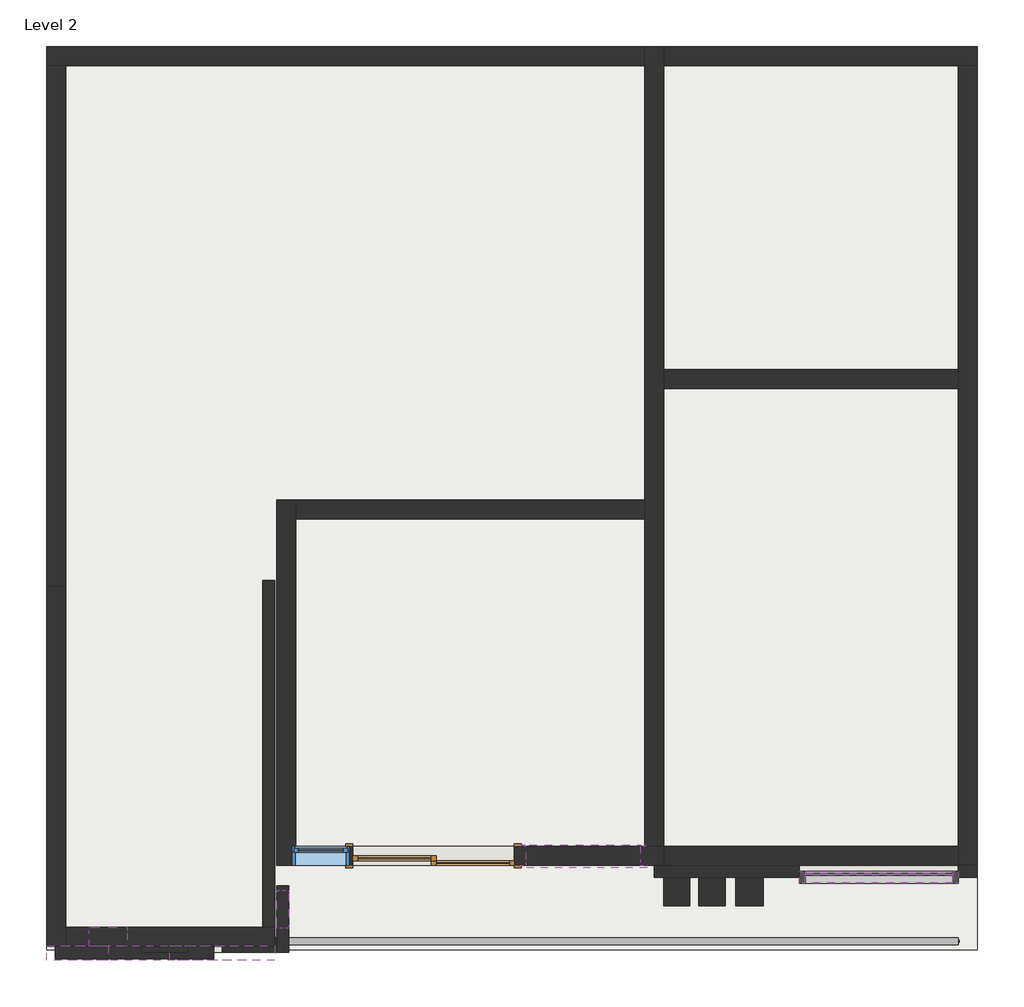
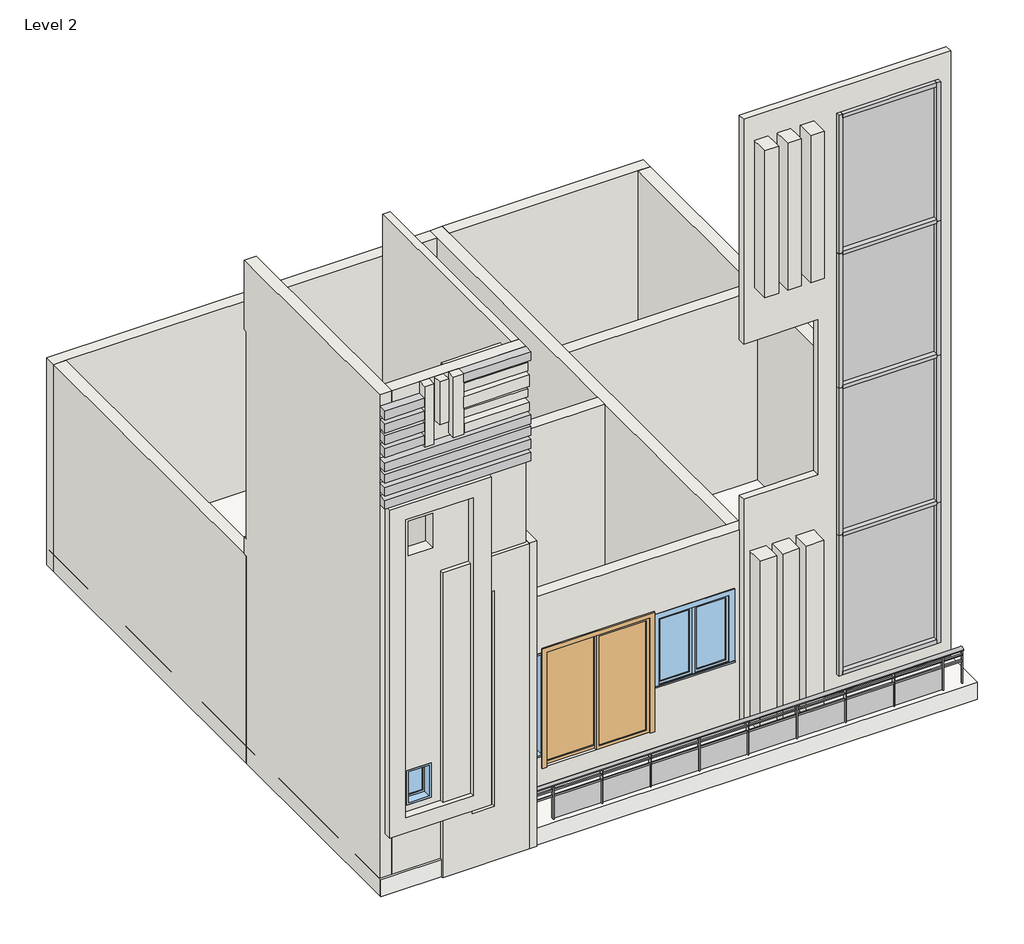
# One storey: 18 walls, 13 members, 9 proxies, 4 plates, 4 windows, 1 door, 1 railing, 1 roof.
"""IFC4 building model written with IfcOpenShell, lengths in millimetres."""

from ifc_helpers import new_model, si_unit, point, frame, origin, place, context, project, spatial, polyline, ellipse_curve, trimmed, outline, extrude, faceted_brep, transform, mapped, element, save
from ifc_brep_helpers import plane_surface, extruded_surface, advanced_brep
from components import door_076b30e0, member_15dc5290, member_cf032248, member_591cd9a7, member_6ce1ec76, member_029677a6, member_d6a8c742, system_panel_glazed_8270a400, system_panel_glazed_e50b416a, system_panel_glazed_3bb4e025, system_panel_glazed_87f78641, walls_3_walls_3_caf9bd33, walls_4_walls_4_15621a10, window_0862ab64, window_085f26e1, window_f83fec05, window_50feeedf

model = new_model("IFC4")

# Units and contexts
model_context = context("Model", 3, world=origin())
ifc_project = project(units=[si_unit("LENGTHUNIT", "METRE", prefix="MILLI")], contexts=[model_context])

# Site, building, storey
site = spatial("IfcSite", under=ifc_project)
building = spatial("IfcBuilding", under=site)
storey = spatial("IfcBuildingStorey", under=building, Name="Level 2", Elevation=3657.6)

# Proxies
placement = place(None, origin())
element("IfcBuildingElementProxy", 1, Name="Cornice", ObjectType="Cornice", at=placement, inside=storey, context=model_context, shape_type="SweptSolid", body=[
    extrude(outline(polyline([(-10979.7013569, 231.2548743), (-10979.7013569, 383.6548743), (-9861.3432037, 383.6548743), (-9861.3432037, 231.2548743), (-10979.7013569, 231.2548743)])), frame((0.0, 0.0, 12344.4), z_axis=(0.0, 0.0, 1.0), x_axis=(1.0, 0.0, 0.0)), (0.0, 0.0, 1.0), 152.4),
])
element("IfcBuildingElementProxy", 2, Name="Cornice", ObjectType="Cornice", at=placement, inside=storey, context=model_context, shape_type="SweptSolid", body=[
    extrude(outline(polyline([(-12299.7432037, 231.2548743), (-12299.7432037, 383.6548743), (-9861.3432037, 383.6548743), (-9861.3432037, 231.2548743), (-12299.7432037, 231.2548743)])), frame((0.0, 0.0, 11226.8), z_axis=(0.0, 0.0, 1.0), x_axis=(1.0, 0.0, 0.0)), (0.0, 0.0, 1.0), 152.4),
])
element("IfcBuildingElementProxy", 3, Name="Cornice", ObjectType="Cornice", at=placement, inside=storey, context=model_context, shape_type="SweptSolid", body=[
    extrude(outline(polyline([(-12299.7432037, 231.2548743), (-12299.7432037, 383.6548743), (-9861.3432037, 383.6548743), (-9861.3432037, 231.2548743), (-12299.7432037, 231.2548743)])), frame((0.0, 0.0, 11023.6), z_axis=(0.0, 0.0, 1.0), x_axis=(1.0, 0.0, 0.0)), (0.0, 0.0, 1.0), 152.4),
])
element("IfcBuildingElementProxy", 4, Name="Cornice", ObjectType="Cornice", at=placement, inside=storey, context=model_context, shape_type="SweptSolid", body=[
    extrude(outline(polyline([(-12299.7432037, 231.2548743), (-12299.7432037, 383.6548743), (-9861.3432037, 383.6548743), (-9861.3432037, 231.2548743), (-12299.7432037, 231.2548743)])), frame((0.0, 0.0, 10795.0), z_axis=(0.0, 0.0, 1.0), x_axis=(1.0, 0.0, 0.0)), (0.0, 0.0, 1.0), 152.4),
])
element("IfcBuildingElementProxy", 5, Name="Cornice", ObjectType="Cornice", at=placement, inside=storey, context=model_context, shape_type="SweptSolid", body=[
    extrude(outline(polyline([(-12299.7432037, 231.2548743), (-12299.7432037, 383.6548743), (-9861.3432037, 383.6548743), (-9861.3432037, 231.2548743), (-12299.7432037, 231.2548743)])), frame((0.0, 0.0, 10566.4), z_axis=(0.0, 0.0, 1.0), x_axis=(1.0, 0.0, 0.0)), (0.0, 0.0, 1.0), 152.4),
])
element("IfcBuildingElementProxy", 6, Name="Cornice", ObjectType="Cornice", at=placement, inside=storey, context=model_context, shape_type="SweptSolid", body=[
    extrude(outline(polyline([(-12299.7432037, 231.2548743), (-12299.7432037, 383.6548743), (-11639.3432037, 383.6548743), (-11639.3432037, 231.2548743), (-12299.7432037, 231.2548743)])), frame((0.0, 0.0, 11480.8), z_axis=(0.0, 0.0, 1.0), x_axis=(1.0, 0.0, 0.0)), (0.0, 0.0, 1.0), 152.4),
])
element("IfcBuildingElementProxy", 7, Name="Cornice", ObjectType="Cornice", at=placement, inside=storey, context=model_context, shape_type="SweptSolid", body=[
    extrude(outline(polyline([(-12299.7432037, 231.2548743), (-12299.7432037, 383.6548743), (-11639.3432037, 383.6548743), (-11639.3432037, 231.2548743), (-12299.7432037, 231.2548743)])), frame((0.0, 0.0, 11709.4), z_axis=(0.0, 0.0, 1.0), x_axis=(1.0, 0.0, 0.0)), (0.0, 0.0, 1.0), 152.4),
])
element("IfcBuildingElementProxy", 8, Name="Cornice", ObjectType="Cornice", at=placement, inside=storey, context=model_context, shape_type="SweptSolid", body=[
    extrude(outline(polyline([(-12299.7432037, 231.2548743), (-12299.7432037, 383.6548743), (-11639.3432037, 383.6548743), (-11639.3432037, 231.2548743), (-12299.7432037, 231.2548743)])), frame((0.0, 0.0, 11912.6), z_axis=(0.0, 0.0, 1.0), x_axis=(1.0, 0.0, 0.0)), (0.0, 0.0, 1.0), 152.4),
])
element("IfcBuildingElementProxy", 9, Name="Cornice", ObjectType="Cornice", at=placement, inside=storey, context=model_context, shape_type="SweptSolid", body=[
    extrude(outline(polyline([(-12299.7432037, 231.2548743), (-12299.7432037, 383.6548743), (-11639.3432037, 383.6548743), (-11639.3432037, 231.2548743), (-12299.7432037, 231.2548743)])), frame((0.0, 0.0, 12141.2), z_axis=(0.0, 0.0, 1.0), x_axis=(1.0, 0.0, 0.0)), (0.0, 0.0, 1.0), 152.4),
])

# Door
door_shape = door_076b30e0(model_context)
element("IfcDoor", 10, ObjectType="Door-Double-Sliding : 68\" x 80\"", at=placement, inside=storey, context=model_context, shape_type="MappedRepresentation", body=[
    mapped(door_shape, transform((-8159.5432037, 1475.8548743, 4267.2), x_axis=(-1.0, 0.0, 0.0), y_axis=(0.0, -1.0, 0.0), z_axis=(0.0, 0.0, 1.0))),
])

# Members
member_shape = member_15dc5290(model_context)
element("IfcMember", 11, ObjectType="Rectangular Mullion : 2.5\" x 5\" rectangular", at=placement, inside=storey, context=model_context, shape_type="MappedRepresentation", body=[
    mapped(member_shape, transform((-4247.9432037, 1120.2548743, 11750.8760868), x_axis=(-1.0, 0.0, 0.0), y_axis=(0.0, -1.0, 0.0), z_axis=(0.0, 0.0, 1.0))),
])
member_2_shape = member_cf032248(model_context)
element("IfcMember", 12, ObjectType="Rectangular Mullion : 2.5\" x 5\" rectangular", at=placement, inside=storey, context=model_context, shape_type="MappedRepresentation", body=[
    mapped(member_2_shape, transform((-4247.9432037, 1120.2548743, 9380.6380434), x_axis=(-1.0, 0.0, 0.0), y_axis=(0.0, -1.0, 0.0), z_axis=(0.0, 0.0, 1.0))),
])
member_3_shape = member_591cd9a7(model_context)
element("IfcMember", 13, ObjectType="Rectangular Mullion : 2.5\" x 5\" rectangular", at=placement, inside=storey, context=model_context, shape_type="MappedRepresentation", body=[
    mapped(member_3_shape, transform((-2609.6432037, 1120.2548743, 11750.8760868), x_axis=(0.0, 0.0, 1.0), y_axis=(0.0, -1.0, 0.0), z_axis=(1.0, 0.0, 0.0))),
])
element("IfcMember", 14, ObjectType="Rectangular Mullion : 2.5\" x 5\" rectangular", at=placement, inside=storey, context=model_context, shape_type="MappedRepresentation", body=[
    mapped(member_3_shape, transform((-2609.6432037, 1120.2548743, 9380.6380434), x_axis=(0.0, 0.0, 1.0), y_axis=(0.0, -1.0, 0.0), z_axis=(1.0, 0.0, 0.0))),
])
element("IfcMember", 15, ObjectType="Rectangular Mullion : 2.5\" x 5\" rectangular", at=placement, inside=storey, context=model_context, shape_type="MappedRepresentation", body=[
    mapped(member_3_shape, transform((-2609.6432037, 1120.2548743, 6781.8), x_axis=(0.0, 0.0, 1.0), y_axis=(0.0, -1.0, 0.0), z_axis=(1.0, 0.0, 0.0))),
])
element("IfcMember", 16, ObjectType="Rectangular Mullion : 2.5\" x 5\" rectangular", at=placement, inside=storey, context=model_context, shape_type="MappedRepresentation", body=[
    mapped(member_shape, transform((-2546.1432037, 1120.2548743, 9380.6380434), x_axis=(1.0, 0.0, 0.0), y_axis=(0.0, -1.0, 0.0), z_axis=(0.0, 0.0, -1.0))),
])
element("IfcMember", 17, ObjectType="Rectangular Mullion : 2.5\" x 5\" rectangular", at=placement, inside=storey, context=model_context, shape_type="MappedRepresentation", body=[
    mapped(member_2_shape, transform((-2546.1432037, 1120.2548743, 6781.8), x_axis=(1.0, 0.0, 0.0), y_axis=(0.0, -1.0, 0.0), z_axis=(0.0, 0.0, -1.0))),
])
member_4_shape = member_6ce1ec76(model_context)
element("IfcMember", 18, ObjectType="Rectangular Mullion : 2.5\" x 5\" rectangular", at=placement, inside=storey, context=model_context, shape_type="MappedRepresentation", body=[
    mapped(member_4_shape, transform((-4184.4432037, 1120.2548743, 4304.5775678), x_axis=(0.0, 0.0, -1.0), y_axis=(0.0, -1.0, 0.0), z_axis=(-1.0, 0.0, 0.0))),
])
member_5_shape = member_029677a6(model_context)
element("IfcMember", 19, ObjectType="Rectangular Mullion : 2.5\" x 5\" rectangular", at=placement, inside=storey, context=model_context, shape_type="MappedRepresentation", body=[
    mapped(member_5_shape, transform((-4247.9432037, 1120.2548743, 6781.8), x_axis=(-1.0, 0.0, 0.0), y_axis=(0.0, -1.0, 0.0), z_axis=(0.0, 0.0, 1.0))),
])
element("IfcMember", 20, ObjectType="Rectangular Mullion : 2.5\" x 5\" rectangular", at=placement, inside=storey, context=model_context, shape_type="MappedRepresentation", body=[
    mapped(member_5_shape, transform((-2546.1432037, 1120.2548743, 4304.5775678), x_axis=(1.0, 0.0, 0.0), y_axis=(0.0, -1.0, 0.0), z_axis=(0.0, 0.0, -1.0))),
])
element("IfcMember", 21, ObjectType="Rectangular Mullion : 2.5\" x 5\" rectangular", at=placement, inside=storey, context=model_context, shape_type="MappedRepresentation", body=[
    mapped(member_4_shape, transform((-2609.6432037, 1120.2548743, 14197.3141302), x_axis=(0.0, 0.0, 1.0), y_axis=(0.0, -1.0, 0.0), z_axis=(1.0, 0.0, 0.0))),
])
member_6_shape = member_d6a8c742(model_context)
element("IfcMember", 22, ObjectType="Rectangular Mullion : 2.5\" x 5\" rectangular", at=placement, inside=storey, context=model_context, shape_type="MappedRepresentation", body=[
    mapped(member_6_shape, transform((-4247.9432037, 1120.2548743, 14197.3141302), x_axis=(-1.0, 0.0, 0.0), y_axis=(0.0, -1.0, 0.0), z_axis=(0.0, 0.0, 1.0))),
])
element("IfcMember", 23, ObjectType="Rectangular Mullion : 2.5\" x 5\" rectangular", at=placement, inside=storey, context=model_context, shape_type="MappedRepresentation", body=[
    mapped(member_6_shape, transform((-2546.1432037, 1120.2548743, 11750.8760868), x_axis=(1.0, 0.0, 0.0), y_axis=(0.0, -1.0, 0.0), z_axis=(0.0, 0.0, -1.0))),
])

# Plates
system_panel_glazed_shape = system_panel_glazed_8270a400(model_context)
element("IfcPlate", 24, ObjectType="System Panel : Glazed", at=placement, inside=storey, context=model_context, shape_type="MappedRepresentation", body=[
    mapped(system_panel_glazed_shape, transform((-3397.0432037, 1120.2548743, 6813.55), x_axis=(1.0, 0.0, 0.0), y_axis=(0.0, 1.0, 0.0), z_axis=(0.0, 0.0, 1.0))),
])
system_panel_glazed_2_shape = system_panel_glazed_e50b416a(model_context)
element("IfcPlate", 25, ObjectType="System Panel : Glazed", at=placement, inside=storey, context=model_context, shape_type="MappedRepresentation", body=[
    mapped(system_panel_glazed_2_shape, transform((-3397.0432037, 1120.2548743, 9412.3880434), x_axis=(1.0, 0.0, 0.0), y_axis=(0.0, 1.0, 0.0), z_axis=(0.0, 0.0, 1.0))),
])
system_panel_glazed_3_shape = system_panel_glazed_3bb4e025(model_context)
element("IfcPlate", 26, ObjectType="System Panel : Glazed", at=placement, inside=storey, context=model_context, shape_type="MappedRepresentation", body=[
    mapped(system_panel_glazed_3_shape, transform((-3397.0432037, 1120.2548743, 4368.0775678), x_axis=(1.0, 0.0, 0.0), y_axis=(0.0, 1.0, 0.0), z_axis=(0.0, 0.0, 1.0))),
])
system_panel_glazed_4_shape = system_panel_glazed_87f78641(model_context)
element("IfcPlate", 27, ObjectType="System Panel : Glazed", at=placement, inside=storey, context=model_context, shape_type="MappedRepresentation", body=[
    mapped(system_panel_glazed_4_shape, transform((-3397.0432037, 1120.2548743, 11782.6260868), x_axis=(1.0, 0.0, 0.0), y_axis=(0.0, 1.0, 0.0), z_axis=(0.0, 0.0, 1.0))),
])

# Railing
element("IfcRailing", 28, ObjectType="Glass Panel - Bottom Fill", at=placement, inside=storey, context=model_context, shape_type="SolidModel", body=[
    advanced_brep(
    [(-9708.9432037, 472.5548476, 4572.0), (-9708.9432037, 396.3548476, 4572.0), (-2546.1432037, 472.5548476, 4572.0), (-2546.1432037, 396.3548476, 4572.0)],
    [
        (0, 1, ellipse_curve(frame((-9708.9432037, 434.4548476, 4572.0), z_axis=(-1.0, 0.0, 0.0), x_axis=(0.0, -1.0, 0.0)), 38.1, 28.575)),
        (1, 0, ellipse_curve(frame((-9708.9432037, 434.4548476, 4572.0), z_axis=(-1.0, 0.0, 0.0), x_axis=(0.0, -1.0, 0.0)), 38.1, 28.575)),
        (2, 3, ellipse_curve(frame((-2546.1432037, 434.4548476, 4572.0), z_axis=(1.0, 0.0, 0.0), x_axis=(0.0, -1.0, 0.0)), 38.1, 28.575)),
        (3, 2, ellipse_curve(frame((-2546.1432037, 434.4548476, 4572.0), z_axis=(1.0, 0.0, 0.0), x_axis=(0.0, -1.0, 0.0)), 38.1, 28.575)),
        (0, 2),
        (3, 1),
    ],
    [
        plane_surface(frame((-9708.9432037, 434.4548476, 4572.0), z_axis=(-1.0, 0.0, 0.0), x_axis=(0.0, 1.0, 0.0))),
        plane_surface(frame((-2546.1432037, 434.4548476, 4572.0), z_axis=(1.0, 0.0, 0.0), x_axis=(0.0, 1.0, 0.0))),
        extruded_surface(trimmed(ellipse_curve(frame((-2546.1432037, 434.4548476, 4572.0), z_axis=(-1.0, 0.0, 0.0), x_axis=(0.0, -1.0, 0.0)), 38.1, 28.575), [point((-2546.1432037, 472.5548476, 4572.0))], [point((-2546.1432037, 396.3548476, 4572.0))], True, "CARTESIAN"), (-7162.800000000001, 0.0, 0.0), 7162.800000000001),
        extruded_surface(trimmed(ellipse_curve(frame((-2546.1432037, 434.4548476, 4572.0), z_axis=(-1.0, 0.0, 0.0), x_axis=(0.0, -1.0, 0.0)), 38.1, 28.575), [point((-2546.1432037, 396.3548476, 4572.0))], [point((-2546.1432037, 472.5548476, 4572.0))], True, "CARTESIAN"), (-7162.800000000001, 0.0, 0.0), 7162.800000000001),
    ],
    [
        (0, [[1, 2]]),
        (1, [[3, 4]]),
        (2, [[-1, 5, -4, 6]]),
        (3, [[-2, -6, -3, -5]]),
    ],
),
    extrude(outline(polyline([(-9708.9432037, 421.7548476), (-9708.9432037, 447.1548476), (-2546.1432037, 447.1548476), (-2546.1432037, 421.7548476), (-9708.9432037, 421.7548476)])), frame((0.0, 0.0, 4457.7), z_axis=(0.0, 0.0, 1.0), x_axis=(1.0, 0.0, 0.0)), (0.0, 0.0, 1.0), 25.4),
    extrude(outline(polyline([(-9708.9432037, 421.7548476), (-9708.9432037, 447.1548476), (-2546.1432037, 447.1548476), (-2546.1432037, 421.7548476), (-9708.9432037, 421.7548476)])), frame((0.0, 0.0, 4356.1), z_axis=(0.0, 0.0, 1.0), x_axis=(1.0, 0.0, 0.0)), (0.0, 0.0, 1.0), 25.4),
    extrude(outline(polyline([(-2882.6932037, 409.0548476), (-2882.6932037, 459.8548476), (-2869.9932037, 459.8548476), (-2869.9932037, 409.0548476), (-2882.6932037, 409.0548476)])), frame((0.0, 0.0, 3657.6), z_axis=(0.0, 0.0, 1.0), x_axis=(1.0, 0.0, 0.0)), (0.0, 0.0, 1.0), 885.6788223),
    extrude(outline(polyline([(-3689.1432037, 440.9900046), (-2876.3432037, 440.9900046), (-2876.3432037, 434.6400046), (-3689.1432037, 434.6400046), (-3689.1432037, 440.9900046)])), frame((0.0, 0.0, 3759.2), z_axis=(0.0, 0.0, 1.0), x_axis=(1.0, 0.0, 0.0)), (0.0, 0.0, 1.0), 596.9),
    extrude(outline(polyline([(-3695.4932037, 409.0548476), (-3695.4932037, 459.8548476), (-3682.7932037, 459.8548476), (-3682.7932037, 409.0548476), (-3695.4932037, 409.0548476)])), frame((0.0, 0.0, 3657.6), z_axis=(0.0, 0.0, 1.0), x_axis=(1.0, 0.0, 0.0)), (0.0, 0.0, 1.0), 885.6788223),
    extrude(outline(polyline([(-4501.9432037, 440.9900046), (-3689.1432037, 440.9900046), (-3689.1432037, 434.6400046), (-4501.9432037, 434.6400046), (-4501.9432037, 440.9900046)])), frame((0.0, 0.0, 3759.2), z_axis=(0.0, 0.0, 1.0), x_axis=(1.0, 0.0, 0.0)), (0.0, 0.0, 1.0), 596.9),
    extrude(outline(polyline([(-4508.2932037, 409.0548476), (-4508.2932037, 459.8548476), (-4495.5932037, 459.8548476), (-4495.5932037, 409.0548476), (-4508.2932037, 409.0548476)])), frame((0.0, 0.0, 3657.6), z_axis=(0.0, 0.0, 1.0), x_axis=(1.0, 0.0, 0.0)), (0.0, 0.0, 1.0), 885.6788223),
    extrude(outline(polyline([(-5314.7432037, 440.9900046), (-4501.9432037, 440.9900046), (-4501.9432037, 434.6400046), (-5314.7432037, 434.6400046), (-5314.7432037, 440.9900046)])), frame((0.0, 0.0, 3759.2), z_axis=(0.0, 0.0, 1.0), x_axis=(1.0, 0.0, 0.0)), (0.0, 0.0, 1.0), 596.9),
    extrude(outline(polyline([(-5321.0932037, 409.0548476), (-5321.0932037, 459.8548476), (-5308.3932037, 459.8548476), (-5308.3932037, 409.0548476), (-5321.0932037, 409.0548476)])), frame((0.0, 0.0, 3657.6), z_axis=(0.0, 0.0, 1.0), x_axis=(1.0, 0.0, 0.0)), (0.0, 0.0, 1.0), 885.6788223),
    extrude(outline(polyline([(-6127.5432037, 440.9900046), (-5314.7432037, 440.9900046), (-5314.7432037, 434.6400046), (-6127.5432037, 434.6400046), (-6127.5432037, 440.9900046)])), frame((0.0, 0.0, 3759.2), z_axis=(0.0, 0.0, 1.0), x_axis=(1.0, 0.0, 0.0)), (0.0, 0.0, 1.0), 596.9),
    extrude(outline(polyline([(-6133.8932037, 409.0548476), (-6133.8932037, 459.8548476), (-6121.1932037, 459.8548476), (-6121.1932037, 409.0548476), (-6133.8932037, 409.0548476)])), frame((0.0, 0.0, 3657.6), z_axis=(0.0, 0.0, 1.0), x_axis=(1.0, 0.0, 0.0)), (0.0, 0.0, 1.0), 885.6788223),
    extrude(outline(polyline([(-6940.3432037, 440.9900046), (-6127.5432037, 440.9900046), (-6127.5432037, 434.6400046), (-6940.3432037, 434.6400046), (-6940.3432037, 440.9900046)])), frame((0.0, 0.0, 3759.2), z_axis=(0.0, 0.0, 1.0), x_axis=(1.0, 0.0, 0.0)), (0.0, 0.0, 1.0), 596.9),
    extrude(outline(polyline([(-6946.6932037, 409.0548476), (-6946.6932037, 459.8548476), (-6933.9932037, 459.8548476), (-6933.9932037, 409.0548476), (-6946.6932037, 409.0548476)])), frame((0.0, 0.0, 3657.6), z_axis=(0.0, 0.0, 1.0), x_axis=(1.0, 0.0, 0.0)), (0.0, 0.0, 1.0), 885.6788223),
    extrude(outline(polyline([(-7753.1432037, 440.9900046), (-6940.3432037, 440.9900046), (-6940.3432037, 434.6400046), (-7753.1432037, 434.6400046), (-7753.1432037, 440.9900046)])), frame((0.0, 0.0, 3759.2), z_axis=(0.0, 0.0, 1.0), x_axis=(1.0, 0.0, 0.0)), (0.0, 0.0, 1.0), 596.9),
    extrude(outline(polyline([(-7759.4932037, 409.0548476), (-7759.4932037, 459.8548476), (-7746.7932037, 459.8548476), (-7746.7932037, 409.0548476), (-7759.4932037, 409.0548476)])), frame((0.0, 0.0, 3657.6), z_axis=(0.0, 0.0, 1.0), x_axis=(1.0, 0.0, 0.0)), (0.0, 0.0, 1.0), 885.6788223),
    extrude(outline(polyline([(-8565.9432037, 440.9900046), (-7753.1432037, 440.9900046), (-7753.1432037, 434.6400046), (-8565.9432037, 434.6400046), (-8565.9432037, 440.9900046)])), frame((0.0, 0.0, 3759.2), z_axis=(0.0, 0.0, 1.0), x_axis=(1.0, 0.0, 0.0)), (0.0, 0.0, 1.0), 596.9),
    extrude(outline(polyline([(-8572.2932037, 409.0548476), (-8572.2932037, 459.8548476), (-8559.5932037, 459.8548476), (-8559.5932037, 409.0548476), (-8572.2932037, 409.0548476)])), frame((0.0, 0.0, 3657.6), z_axis=(0.0, 0.0, 1.0), x_axis=(1.0, 0.0, 0.0)), (0.0, 0.0, 1.0), 885.6788223),
    extrude(outline(polyline([(-9378.7432037, 440.9900046), (-8565.9432037, 440.9900046), (-8565.9432037, 434.6400046), (-9378.7432037, 434.6400046), (-9378.7432037, 440.9900046)])), frame((0.0, 0.0, 3759.2), z_axis=(0.0, 0.0, 1.0), x_axis=(1.0, 0.0, 0.0)), (0.0, 0.0, 1.0), 596.9),
    extrude(outline(polyline([(-9385.0932037, 409.0548476), (-9385.0932037, 459.8548476), (-9372.3932037, 459.8548476), (-9372.3932037, 409.0548476), (-9385.0932037, 409.0548476)])), frame((0.0, 0.0, 3657.6), z_axis=(0.0, 0.0, 1.0), x_axis=(1.0, 0.0, 0.0)), (0.0, 0.0, 1.0), 885.6788223),
    extrude(outline(polyline([(-2558.8432037, 424.9298476), (-2558.8432037, 443.9798476), (-2539.7932037, 443.9798476), (-2539.7932037, 424.9298476), (-2558.8432037, 424.9298476)])), frame((0.0, 0.0, 3657.6), z_axis=(0.0, 0.0, 1.0), x_axis=(1.0, 0.0, 0.0)), (0.0, 0.0, 1.0), 885.6788223),
    extrude(outline(polyline([(-9715.2932037, 424.9298476), (-9715.2932037, 443.9798476), (-9696.2432037, 443.9798476), (-9696.2432037, 424.9298476), (-9715.2932037, 424.9298476)])), frame((0.0, 0.0, 3657.6), z_axis=(0.0, 0.0, 1.0), x_axis=(1.0, 0.0, 0.0)), (0.0, 0.0, 1.0), 885.6788223),
])

# Roof
element("IfcRoof", 29, ObjectType="Generic - 12\"", at=placement, inside=storey, context=model_context, shape_type="SweptSolid", body=[
    extrude(outline(polyline([(-12299.7432037, 10010.2548743), (-2342.9432037, 10010.2548743), (-2342.9432037, 345.6498736), (-12299.7432037, 345.6498736), (-12299.7432037, 10010.2548743)])), frame((0.0, 0.0, 3657.6), z_axis=(0.0, 0.0, 1.0), x_axis=(1.0, 0.0, 0.0)), (0.0, 0.0, 1.0), 304.8),
])

# Walls
element("IfcWall", 30, ObjectType="Generic - 5\"", at=placement, inside=storey, context=model_context, shape_type="Brep", body=[
    faceted_brep([(-9835.9432037, 1031.3548743, 3657.6), (-9835.9432037, 472.5548476, 3657.6), (-9835.9432037, 320.1548476, 3657.6), (-9835.9432037, 320.1548476, 9041.1857602), (-9835.9432037, 320.1548476, 9049.6221659), (-9835.9432037, 1031.3548743, 9049.6221659), (-9835.9432037, 980.5548743, 7155.1038477), (-9835.9432037, 574.1548743, 7155.1038477), (-9835.9432037, 574.1548743, 5935.9038477), (-9835.9432037, 980.5548743, 5935.9038477), (-9708.9432037, 1031.3548743, 3657.6), (-9708.9432037, 1031.3548743, 9049.6221659), (-9708.9432037, 320.1548476, 9049.6221659), (-9708.9432037, 320.1548476, 3657.6), (-9708.9432037, 980.5548743, 7155.1038477), (-9708.9432037, 980.5548743, 5935.9038477), (-9708.9432037, 574.1548743, 5935.9038477), (-9708.9432037, 574.1548743, 7155.1038477)], [[[0, 1, 2, 3, 4, 5], [6, 7, 8, 9]], [[10, 11, 12, 13], [14, 15, 16, 17]], [[2, 1, 0, 10, 13]], [[5, 4, 12, 11]], [[0, 5, 11, 10]], [[4, 3, 2, 13, 12]], [[15, 14, 6, 9]], [[16, 15, 9, 8]], [[17, 16, 8, 7]], [[14, 17, 7, 6]]]),
])
element("IfcWall", 31, ObjectType="Generic - 5\"", at=placement, inside=storey, context=model_context, shape_type="Brep", body=[
    faceted_brep([(-9861.3432037, 586.8548743, 3657.6), (-9861.3432037, 4295.2548743, 3657.6), (-9861.3432037, 4295.2548743, 12496.8), (-9861.3432037, 586.8548743, 12496.8), (-9861.3432037, 1158.3548743, 10314.2841054), (-9861.3432037, 1158.3548743, 9095.0841054), (-9861.3432037, 751.9548743, 9095.0841054), (-9861.3432037, 751.9548743, 10314.2841054), (-9988.3432037, 4295.2548743, 3657.6), (-9988.3432037, 586.8548743, 3657.6), (-9988.3432037, 586.8548743, 12496.8), (-9988.3432037, 4168.2548743, 12496.8), (-9988.3432037, 4295.2548743, 12496.8), (-9988.3432037, 4295.2548743, 7315.2), (-9988.3432037, 1158.3548743, 9095.0841054), (-9988.3432037, 1158.3548743, 10314.2841054), (-9988.3432037, 751.9548743, 10314.2841054), (-9988.3432037, 751.9548743, 9095.0841054)], [[[0, 1, 2, 3], [4, 5, 6, 7]], [[8, 9, 10, 11, 12, 13], [14, 15, 16, 17]], [[1, 0, 9, 8]], [[3, 2, 12, 11, 10]], [[0, 3, 10, 9]], [[2, 1, 8, 13, 12]], [[5, 4, 15, 14]], [[6, 5, 14, 17]], [[7, 6, 17, 16]], [[4, 7, 16, 15]]]),
])
element("IfcWall", 32, ObjectType="Generic - 5\"", at=placement, inside=storey, context=model_context, shape_type="SweptSolid", body=[
    extrude(outline(polyline([(3657.6, -2342.9432037), (14630.4, -2342.9432037), (14630.4, -5797.3432037), (10668.0, -5797.3432037), (10668.0, -4552.7432037), (7924.8, -4552.7432037), (7924.8, -5797.3432037), (3657.6, -5797.3432037), (3657.6, -2342.9432037)]), holes=[polyline([(11277.6, -4247.9432037), (14197.3141302, -4247.9432037), (14197.3141302, -2546.1432037), (11277.6, -2546.1432037), (4304.5775678, -2546.1432037), (4304.5775678, -4247.9432037), (11277.6, -4247.9432037)])]), frame((0.0, 1120.2548743, 0.0), z_axis=(0.0, 1.0, 0.0), x_axis=(0.0, 0.0, 1.0)), (0.0, 0.0, 1.0), 127.0),
])
element("IfcWall", 33, ObjectType="Generic - 6\"", at=placement, inside=storey, context=model_context, shape_type="SweptSolid", body=[
    extrude(outline(polyline([(3657.6, -9835.9432037), (9041.1857602, -9835.9432037), (9041.1857602, -11283.7432037), (3657.6, -11283.7432037), (3657.6, -9835.9432037)]), holes=[polyline([(8420.1676398, -10420.1432037), (4614.2361055, -10420.1432037), (4614.2361055, -10790.5776586), (8420.1676398, -10790.5776586), (8420.1676398, -10420.1432037)])]), frame((0.0, 320.1548476, 0.0), z_axis=(0.0, 1.0, 0.0), x_axis=(0.0, 0.0, 1.0)), (0.0, 0.0, 1.0), 152.4),
])
element("IfcWall", 34, ObjectType="Generic - 8\"", at=placement, inside=storey, context=model_context, shape_type="Brep", body=[
    faceted_brep([(-9835.9432037, 5158.8548743, 3657.6), (-9835.9432037, 1247.2548743, 3657.6), (-9835.9432037, 1247.2548743, 7315.2), (-9835.9432037, 5158.8548743, 7315.2), (-9632.7432037, 1247.2548743, 3657.6), (-9632.7432037, 1450.4548743, 3657.6), (-9632.7432037, 4955.6548743, 3657.6), (-9632.7432037, 5158.8548743, 3657.6), (-9632.7432037, 5158.8548743, 7315.2), (-9632.7432037, 4955.6548743, 7315.2), (-9632.7432037, 1450.4548743, 7315.2), (-9632.7432037, 1247.2548743, 7315.2), (-9632.7432037, 1247.2548743, 6297.883541), (-9632.7432037, 1450.4548743, 6297.883541), (-9632.7432037, 1450.4548743, 4469.083541), (-9632.7432037, 1247.2548743, 4469.083541), (-9670.8432037, 1247.2548743, 4469.083541), (-9670.8432037, 1247.2548743, 6297.883541), (-9670.8432037, 1450.4548743, 6297.883541), (-9670.8432037, 1450.4548743, 4469.083541)], [[[0, 1, 2, 3]], [[4, 5, 6, 7, 8, 9, 10, 11, 12, 13, 14, 15]], [[1, 0, 7, 6, 5, 4]], [[3, 2, 11, 10, 9, 8]], [[2, 1, 4, 15, 16, 17, 12, 11]], [[0, 3, 8, 7]], [[18, 19, 14, 13]], [[19, 16, 15, 14]], [[19, 18, 17, 16]], [[17, 18, 13, 12]]]),
])
element("IfcWall", 35, ObjectType="Generic - 8\"", at=placement, inside=storey, context=model_context, shape_type="Brep", body=[
    faceted_brep([(-9632.7432037, 1247.2548743, 3657.6), (-5695.7432037, 1247.2548743, 3657.6), (-5695.7432037, 1247.2548743, 7315.2), (-9632.7432037, 1247.2548743, 7315.2), (-9632.7432037, 1247.2548743, 6297.883541), (-9061.2432037, 1247.2548743, 6297.883541), (-9061.2432037, 1247.2548743, 4469.083541), (-9632.7432037, 1247.2548743, 4469.083541), (-7295.9432037, 1247.2548743, 6299.2), (-7295.9432037, 1247.2548743, 4267.2), (-9023.1432037, 1247.2548743, 4267.2), (-9023.1432037, 1247.2548743, 6299.2), (-7168.9432037, 1247.2548743, 5024.3797093), (-7168.9432037, 1247.2548743, 6243.5797093), (-5949.7432037, 1247.2548743, 6243.5797093), (-5949.7432037, 1247.2548743, 5024.3797093), (-5695.7432037, 1450.4548743, 3657.6), (-5898.9432037, 1450.4548743, 3657.6), (-9632.7432037, 1450.4548743, 3657.6), (-9632.7432037, 1450.4548743, 4469.083541), (-9061.2432037, 1450.4548743, 4469.083541), (-9061.2432037, 1450.4548743, 6297.883541), (-9632.7432037, 1450.4548743, 6297.883541), (-9632.7432037, 1450.4548743, 7315.2), (-5898.9432037, 1450.4548743, 7315.2), (-5695.7432037, 1450.4548743, 7315.2), (-7295.9432037, 1450.4548743, 4267.2), (-7295.9432037, 1450.4548743, 6299.2), (-9023.1432037, 1450.4548743, 6299.2), (-9023.1432037, 1450.4548743, 4267.2), (-7168.9432037, 1450.4548743, 6243.5797093), (-7168.9432037, 1450.4548743, 5024.3797093), (-5949.7432037, 1450.4548743, 5024.3797093), (-5949.7432037, 1450.4548743, 6243.5797093)], [[[0, 1, 2, 3, 4, 5, 6, 7], [8, 9, 10, 11], [12, 13, 14, 15]], [[16, 17, 18, 19, 20, 21, 22, 23, 24, 25], [26, 27, 28, 29], [30, 31, 32, 33]], [[1, 0, 18, 17, 16]], [[3, 2, 25, 24, 23]], [[3, 23, 22, 4]], [[18, 0, 7, 19]], [[2, 1, 16, 25]], [[8, 27, 26, 9]], [[10, 29, 28, 11]], [[27, 8, 11, 28]], [[29, 10, 9, 26]], [[31, 30, 13, 12]], [[32, 31, 12, 15]], [[33, 32, 15, 14]], [[30, 33, 14, 13]], [[5, 21, 20, 6]], [[7, 6, 20, 19]], [[21, 5, 4, 22]]]),
])
element("IfcWall", 36, ObjectType="Generic - 8\"", at=placement, inside=storey, context=model_context, shape_type="Brep", body=[
    faceted_brep([(-5695.7432037, 1450.4548743, 3657.6), (-5695.7432037, 6352.6548743, 3657.6), (-5695.7432037, 6555.8548743, 3657.6), (-5695.7432037, 9807.0548743, 3657.6), (-5695.7432037, 10010.2548743, 3657.6), (-5695.7432037, 10010.2548743, 7315.2), (-5695.7432037, 9807.0548743, 7315.2), (-5695.7432037, 6555.8548743, 7315.2), (-5695.7432037, 6352.6548743, 7315.2), (-5695.7432037, 1450.4548743, 7315.2), (-5898.9432037, 1450.4548743, 3657.6), (-5898.9432037, 1450.4548743, 7315.2), (-5898.9432037, 4955.6548743, 7315.2), (-5898.9432037, 5158.8548743, 7315.2), (-5898.9432037, 9807.0548743, 7315.2), (-5898.9432037, 10010.2548743, 7315.2), (-5898.9432037, 10010.2548743, 3657.6), (-5898.9432037, 9807.0548743, 3657.6), (-5898.9432037, 5158.8548743, 3657.6), (-5898.9432037, 4955.6548743, 3657.6)], [[[0, 1, 2, 3, 4, 5, 6, 7, 8, 9]], [[10, 11, 12, 13, 14, 15, 16, 17, 18, 19]], [[4, 3, 2, 1, 0, 10, 19, 18, 17, 16]], [[9, 8, 7, 6, 5, 15, 14, 13, 12, 11]], [[0, 9, 11, 10]], [[5, 4, 16, 15]]]),
])
element("IfcWall", 37, ObjectType="Generic - 8\"", at=placement, inside=storey, context=model_context, shape_type="SweptSolid", body=[
    extrude(outline(polyline([(-2546.1432037, 6352.6548743), (-5695.7432037, 6352.6548743), (-5695.7432037, 6555.8548743), (-2546.1432037, 6555.8548743), (-2546.1432037, 6352.6548743)])), frame((0.0, 0.0, 3657.6), z_axis=(0.0, 0.0, 1.0), x_axis=(1.0, 0.0, 0.0)), (0.0, 0.0, 1.0), 3657.6),
])
element("IfcWall", 38, ObjectType="Generic - 8\"", at=placement, inside=storey, context=model_context, shape_type="Brep", body=[
    faceted_brep([(-12299.7432037, 4231.7548743, 3657.6), (-12299.7432037, 383.6548743, 3657.6), (-12299.7432037, 383.6548743, 9093.2), (-12299.7432037, 383.6548743, 9245.6), (-12299.7432037, 383.6548743, 12496.8), (-12299.7432037, 4295.2548743, 12496.8), (-12299.7432037, 4295.2548743, 11277.6), (-12299.7432037, 4231.7548743, 11277.6), (-12299.7432037, 4231.7548743, 7620.0), (-12299.7432037, 4295.2548743, 7620.0), (-12299.7432037, 4295.2548743, 7315.2), (-12299.7432037, 4231.7548743, 7315.2), (-12096.5432037, 383.6548743, 3657.6), (-12096.5432037, 586.8548743, 3657.6), (-12096.5432037, 4231.7548743, 3657.6), (-12096.5432037, 4231.7548743, 7315.2), (-12096.5432037, 4295.2548743, 7315.2), (-12096.5432037, 4295.2548743, 7620.0), (-12096.5432037, 4231.7548743, 7620.0), (-12096.5432037, 4231.7548743, 11277.6), (-12096.5432037, 4295.2548743, 11277.6), (-12096.5432037, 4295.2548743, 12496.8), (-12096.5432037, 4168.2548743, 12496.8), (-12096.5432037, 586.8548743, 12496.8), (-12096.5432037, 383.6548743, 12496.8), (-12096.5432037, 383.6548743, 9245.6), (-12096.5432037, 383.6548743, 9093.2)], [[[0, 1, 2, 3, 4, 5, 6, 7, 8, 9, 10, 11]], [[12, 13, 14, 15, 16, 17, 18, 19, 20, 21, 22, 23, 24, 25, 26]], [[1, 0, 14, 13, 12]], [[5, 4, 24, 23, 22, 21]], [[1, 12, 26, 25, 24, 4, 3, 2]], [[14, 0, 11, 15]], [[16, 15, 11, 10]], [[8, 18, 17, 9]], [[18, 8, 7, 19]], [[20, 19, 7, 6]], [[10, 9, 17, 16]], [[6, 5, 21, 20]]]),
])
element("IfcWall", 39, ObjectType="Generic - 8\"", at=placement, inside=storey, context=model_context, shape_type="Brep", body=[
    faceted_brep([(-12096.5432037, 383.6548743, 3657.6), (-9861.3432037, 383.6548743, 3657.6), (-9861.3432037, 383.6548743, 12496.8), (-12096.5432037, 383.6548743, 12496.8), (-11436.1432037, 383.6548743, 5703.493049), (-11436.1432037, 383.6548743, 5093.893049), (-11842.5432037, 383.6548743, 5093.893049), (-11842.5432037, 383.6548743, 5703.493049), (-11410.7432037, 383.6548743, 10095.2555904), (-11410.7432037, 383.6548743, 9485.6555904), (-11817.1432037, 383.6548743, 9485.6555904), (-11817.1432037, 383.6548743, 10095.2555904), (-12096.5432037, 586.8548743, 3657.6), (-12096.5432037, 586.8548743, 12496.8), (-9988.3432037, 586.8548743, 12496.8), (-9861.3432037, 586.8548743, 12496.8), (-9861.3432037, 586.8548743, 3657.6), (-9988.3432037, 586.8548743, 3657.6), (-11436.1432037, 586.8548743, 5703.493049), (-11842.5432037, 586.8548743, 5703.493049), (-11842.5432037, 586.8548743, 5093.893049), (-11436.1432037, 586.8548743, 5093.893049), (-11410.7432037, 586.8548743, 10095.2555904), (-11817.1432037, 586.8548743, 10095.2555904), (-11817.1432037, 586.8548743, 9485.6555904), (-11410.7432037, 586.8548743, 9485.6555904)], [[[0, 1, 2, 3], [4, 5, 6, 7], [8, 9, 10, 11]], [[12, 13, 14, 15, 16, 17], [18, 19, 20, 21], [22, 23, 24, 25]], [[1, 0, 12, 17, 16]], [[3, 2, 15, 14, 13]], [[0, 3, 13, 12]], [[2, 1, 16, 15]], [[5, 4, 18, 21]], [[6, 5, 21, 20]], [[7, 6, 20, 19]], [[4, 7, 19, 18]], [[9, 8, 22, 25]], [[10, 9, 25, 24]], [[11, 10, 24, 23]], [[8, 11, 23, 22]]]),
])
element("IfcWall", 40, ObjectType="Generic - 8\"", at=placement, inside=storey, context=model_context, shape_type="Brep", body=[
    faceted_brep([(-2546.1432037, 9807.0548743, 3657.6), (-2546.1432037, 6555.8548743, 3657.6), (-2546.1432037, 6352.6548743, 3657.6), (-2546.1432037, 1450.4548743, 3657.6), (-2546.1432037, 1247.2548743, 3657.6), (-2546.1432037, 1247.2548743, 7315.2), (-2546.1432037, 1450.4548743, 7315.2), (-2546.1432037, 6352.6548743, 7315.2), (-2546.1432037, 6555.8548743, 7315.2), (-2546.1432037, 9807.0548743, 7315.2), (-2342.9432037, 9807.0548743, 3657.6), (-2342.9432037, 9807.0548743, 7315.2), (-2342.9432037, 1247.2548743, 7315.2), (-2342.9432037, 1247.2548743, 3657.6)], [[[0, 1, 2, 3, 4, 5, 6, 7, 8, 9]], [[10, 11, 12, 13]], [[4, 3, 2, 1, 0, 10, 13]], [[9, 8, 7, 6, 5, 12, 11]], [[5, 4, 13, 12]], [[0, 9, 11, 10]]]),
])
element("IfcWall", 41, ObjectType="Generic - 8\"", at=placement, inside=storey, context=model_context, shape_type="SweptSolid", body=[
    extrude(outline(polyline([(-2546.1432037, 1247.2548743), (-5695.7432037, 1247.2548743), (-5695.7432037, 1450.4548743), (-2546.1432037, 1450.4548743), (-2546.1432037, 1247.2548743)])), frame((0.0, 0.0, 3657.6), z_axis=(0.0, 0.0, 1.0), x_axis=(1.0, 0.0, 0.0)), (0.0, 0.0, 1.0), 3657.6),
])
element("IfcWall", 42, ObjectType="Generic - 8\"", at=placement, inside=storey, context=model_context, shape_type="SweptSolid", body=[
    extrude(outline(polyline([(-5898.9432037, 4955.6548743), (-9632.7432037, 4955.6548743), (-9632.7432037, 5158.8548743), (-5898.9432037, 5158.8548743), (-5898.9432037, 4955.6548743)])), frame((0.0, 0.0, 3657.6), z_axis=(0.0, 0.0, 1.0), x_axis=(1.0, 0.0, 0.0)), (0.0, 0.0, 1.0), 3657.6),
])
element("IfcWall", 43, ObjectType="Generic - 8\"", at=placement, inside=storey, context=model_context, shape_type="Brep", body=[
    faceted_brep([(-5898.9432037, 10010.2548743, 3657.6), (-12299.7432037, 10010.2548743, 3657.6), (-12299.7432037, 10010.2548743, 7315.2), (-5898.9432037, 10010.2548743, 7315.2), (-5898.9432037, 9807.0548743, 3657.6), (-5898.9432037, 9807.0548743, 7315.2), (-12096.5432037, 9807.0548743, 7315.2), (-12299.7432037, 9807.0548743, 7315.2), (-12299.7432037, 9807.0548743, 3657.6), (-12096.5432037, 9807.0548743, 3657.6)], [[[0, 1, 2, 3]], [[4, 5, 6, 7, 8, 9]], [[1, 0, 4, 9, 8]], [[3, 2, 7, 6, 5]], [[0, 3, 5, 4]], [[2, 1, 8, 7]]]),
])
element("IfcWall", 44, ObjectType="Generic - 8\"", at=placement, inside=storey, context=model_context, shape_type="Brep", body=[
    faceted_brep([(-12299.7432037, 9807.0548743, 3657.6), (-12299.7432037, 4231.7548743, 3657.6), (-12299.7432037, 4231.7548743, 7315.2), (-12299.7432037, 4295.2548743, 7315.2), (-12299.7432037, 9807.0548743, 7315.2), (-12096.5432037, 9807.0548743, 3657.6), (-12096.5432037, 9807.0548743, 7315.2), (-12096.5432037, 4295.2548743, 7315.2), (-12096.5432037, 4231.7548743, 7315.2), (-12096.5432037, 4231.7548743, 3657.6)], [[[0, 1, 2, 3, 4]], [[5, 6, 7, 8, 9]], [[1, 0, 5, 9]], [[2, 1, 9, 8]], [[4, 3, 2, 8, 7, 6]], [[0, 4, 6, 5]]]),
])
element("IfcWall", 45, ObjectType="Generic - 8\"", at=placement, inside=storey, context=model_context, shape_type="Brep", body=[
    faceted_brep([(-5695.7432037, 9807.0548743, 3657.6), (-2546.1432037, 9807.0548743, 3657.6), (-2342.9432037, 9807.0548743, 3657.6), (-2342.9432037, 9807.0548743, 7315.2), (-2546.1432037, 9807.0548743, 7315.2), (-5695.7432037, 9807.0548743, 7315.2), (-5695.7432037, 10010.2548743, 3657.6), (-5695.7432037, 10010.2548743, 7315.2), (-2342.9432037, 10010.2548743, 7315.2), (-2342.9432037, 10010.2548743, 3657.6)], [[[0, 1, 2, 3, 4, 5]], [[6, 7, 8, 9]], [[2, 1, 0, 6, 9]], [[5, 4, 3, 8, 7]], [[0, 5, 7, 6]], [[3, 2, 9, 8]]]),
])
walls_3_walls_3_shape = walls_3_walls_3_caf9bd33(model_context)
element("IfcWall", 46, ObjectType="Walls 3 : Walls 3", at=placement, inside=storey, context=model_context, shape_type="MappedRepresentation", body=[
    mapped(walls_3_walls_3_shape, transform((0.0, 0.0, 0.0), x_axis=(1.0, 0.0, 0.0), y_axis=(0.0, 1.0, 0.0), z_axis=(0.0, 0.0, 1.0))),
])
walls_4_walls_4_shape = walls_4_walls_4_15621a10(model_context)
element("IfcWall", 47, ObjectType="Walls 4 : Walls 4", at=placement, inside=storey, context=model_context, shape_type="MappedRepresentation", body=[
    mapped(walls_4_walls_4_shape, transform((0.0, 0.0, 0.0), x_axis=(1.0, 0.0, 0.0), y_axis=(0.0, 1.0, 0.0), z_axis=(0.0, 0.0, 1.0))),
])

# Windows
window_shape = window_0862ab64(model_context)
element("IfcWindow", 48, ObjectType="Casement Dbl with Trim : 48\" x 48\"", at=placement, inside=storey, context=model_context, shape_type="MappedRepresentation", body=[
    mapped(window_shape, transform((-6559.3432037, 1367.9048743, 4109.9797093), x_axis=(-1.0, 0.0, 0.0), y_axis=(0.0, -1.0, 0.0), z_axis=(0.0, 0.0, 1.0))),
])
window_2_shape = window_085f26e1(model_context)
element("IfcWindow", 49, ObjectType="Fixed : 16\" x 24\"", at=placement, inside=storey, context=model_context, shape_type="MappedRepresentation", body=[
    mapped(window_2_shape, transform((-11601.2432037, 485.2548743, 4179.493049), x_axis=(1.0, 0.0, 0.0), y_axis=(0.0, 1.0, 0.0), z_axis=(0.0, 0.0, 1.0))),
])
window_3_shape = window_f83fec05(model_context)
element("IfcWindow", 50, ObjectType="Fixed : 16\" x 48\"", at=placement, inside=storey, context=model_context, shape_type="MappedRepresentation", body=[
    mapped(window_3_shape, transform((-9772.4432037, 815.4548743, 5021.5038477), x_axis=(0.0, 1.0, 0.0), y_axis=(-1.0, 0.0, 0.0), z_axis=(0.0, 0.0, 1.0))),
])
window_4_shape = window_50feeedf(model_context)
element("IfcWindow", 51, ObjectType="Fixed : 24\" x 72\"", at=placement, inside=storey, context=model_context, shape_type="MappedRepresentation", body=[
    mapped(window_4_shape, transform((-9327.9432037, 1348.8548743, 4164.283541), x_axis=(1.0, 0.0, 0.0), y_axis=(0.0, 1.0, 0.0), z_axis=(0.0, 0.0, 1.0))),
])

save(model, "model.ifc")

# Revit data of these elements
# Type "Door-Double-Sliding : 68\" x 80\""
#   Type Mark = "8"
#   Construction Type Id = "opn-d45"
#   Assembly Code = "C1020"
#   Analytic Construction = "Wood frame, double glass door "
#   Thickness = 0' - 2"
#   Thermal Resistance (R) = 1.8150 (h·ft²·°F)/BTU
#   Heat Transfer Coefficient (U) = 0.5510 BTU/(h·ft²·°F)
#   Height = 6' - 8"
#   Rail Width = 0' - 2"
#   Stiles = 0' - 2"
#   Trim Projection Ext = 0' - 1"
#   Trim Projection Int = 0' - 1"
#   Trim Width = 0' - 3"
#   Width = 5' - 8"
#   Define Thermal Properties by = 1
#   Glazing = Glass
#   Panel Material = Wood - Birch - Solid Stained Light Low Gloss
#   Trim Material = Paint - Sienna
#   Visual Light Transmittance = 0
#   Solar Heat Gain Coefficient = 0
#   Function = (empty or 0)
#   Wall Closure = (empty or 0)
# Type "Rectangular Mullion : 2.5\" x 5\" rectangular"
#   built-in parameter 1007304 = 0.416667 (stored number, unit not read)
#   built-in parameter 1007301 = 0.104167 (stored number, unit not read)
#   built-in parameter 1007300 = 0.104167 (stored number, unit not read)
# Type "System Panel : Glazed"
#   Construction Type Id = "GSP4R"
#   Analytic Construction = "1/8 in Pilkington single glazing"
#   Visual Light Transmittance = 0.9
#   Solar Heat Gain Coefficient = 0.86
#   Heat Transfer Coefficient (U) = 1.18115 BTU/(h·ft²·°F)
# Type "Glass Panel - Bottom Fill"
#   Assembly Code = "C2010400"
#   built-in parameter 1008612 = 0.0416667 (stored number, unit not read)
#   built-in parameter 1008611 = 0.0416667 (stored number, unit not read)
#   built-in parameter 1008609 = 0.333333 (stored number, unit not read)
#   built-in parameter 1008604 = 0.166667 (stored number, unit not read)
#   built-in parameter 1008603 = 0.166667 (stored number, unit not read)
#   Railing Height = 3' - 0"
#   built-in parameter 1008630 = 2
#   built-in parameter 1008610 = 2
#   built-in parameter 1008618 = Baluster - Square : 3/4"
# Type "Generic - 12\""
#   Assembly Code = "B1020"
#   Layers, outside or top first: 1' - 0" no material (function 1)
# Type "Generic - 5\""
#   Assembly Code = "B2010"
#   Layers, outside or top first: 0' - 5" no material (function 1)
# Type "Generic - 6\""
#   Assembly Code = "B2010"
#   Layers, outside or top first: 0' - 6" no material (function 1)
# Type "Generic - 8\""
#   Assembly Code = "B2010"
#   Layers, outside or top first: 0' - 8" no material (function 1)
# Type "Casement Dbl with Trim : 48\" x 48\""
#   Type Mark = "13"
#   Construction Type Id = "GSP4R"
#   Assembly Code = "B2020100"
#   Analytic Construction = "1/8 in Pilkington single glazing"
#   Visual Light Transmittance = 0.9
#   Thermal Resistance (R) = 1.53941 (h·ft²·°F)/BTU
#   Solar Heat Gain Coefficient = 0.78
#   Heat Transfer Coefficient (U) = 0.6496 BTU/(h·ft²·°F)
#   Height = 4' - 0"
#   Default Sill Height = 3' - 0"
#   Trim Projection - Ext. = 0' - 0 1/2"
#   Trim Projection - Int. = 0' - 0 3/4"
#   Trim Width - Exterior = 0' - 3 1/2"
#   Trim Width - Interior = 0' - 3 1/2"
#   Width = 4' - 0"
#   Window Inset = 0' - 0 3/4"
#   Define Thermal Properties by = 1
#   Glass Pane Material = Glass
#   Sash Material = Sash
#   Trim Exterior Material = Trim
#   Trim Interior Material = Trim
#   Wall Closure = (empty or 0)
# Type "Fixed : 16\" x 24\""
#   Type Mark = "4"
#   Construction Type Id = "GSP4R"
#   Assembly Code = "B2020100"
#   Analytic Construction = "1/8 in Pilkington single glazing"
#   Visual Light Transmittance = 0.9
#   Solar Heat Gain Coefficient = 0.78
#   Heat Transfer Coefficient (U) = 0.6496 BTU/(h·ft²·°F)
#   Height = 2' - 0"
#   Default Sill Height = 3' - 0"
#   Width = 1' - 4"
#   Window Inset = 0' - 0 3/4"
#   Define Thermal Properties by = 1
#   Glass Pane Material = Glass
#   Sash Material = Sash
#   Wall Closure = (empty or 0)
# Type "Fixed : 16\" x 48\""
#   Type Mark = "5"
#   Construction Type Id = "GSP4R"
#   Assembly Code = "B2020100"
#   Analytic Construction = "1/8 in Pilkington single glazing"
#   Visual Light Transmittance = 0.9
#   Solar Heat Gain Coefficient = 0.78
#   Heat Transfer Coefficient (U) = 0.6496 BTU/(h·ft²·°F)
#   Height = 4' - 0"
#   Default Sill Height = 3' - 0"
#   Width = 1' - 4"
#   Window Inset = 0' - 0 3/4"
#   Define Thermal Properties by = 1
#   Glass Pane Material = Glass
#   Sash Material = Sash
#   Wall Closure = (empty or 0)
# Type "Fixed : 24\" x 72\""
#   Type Mark = "7"
#   Construction Type Id = "GSP4R"
#   Assembly Code = "B2020100"
#   Analytic Construction = "1/8 in Pilkington single glazing"
#   Visual Light Transmittance = 0.9
#   Solar Heat Gain Coefficient = 0.78
#   Heat Transfer Coefficient (U) = 0.6496 BTU/(h·ft²·°F)
#   Height = 6' - 0"
#   Default Sill Height = 1' - 0"
#   Width = 2' - 0"
#   Window Inset = 0' - 0 3/4"
#   Define Thermal Properties by = 1
#   Glass Pane Material = Glass
#   Sash Material = Sash
#   Wall Closure = (empty or 0)
# Elements 1, 2, 3, 4, 5, 6, 7, 8, 9 (IfcBuildingElementProxy, "Cornice")
#   Phase Created = New Construction
#   Materials on its faces: "Default Wall"
# Element 10 (IfcDoor, "Door-Double-Sliding : 68\" x 80\"")
#   Phase Created = New Construction
#   Materials on its faces: "Paint - Sienna", "Wood - Birch - Solid Stained Light Low Gloss", "Glass"
# Elements 11, 12, 13, 14, 15, 16, 17, 18, 19, 20, 21, 22, 23 (IfcMember, "Rectangular Mullion : 2.5\" x 5\" rectangular")
#   Phase Created = New Construction
#   Materials on its faces: "Aluminum"
# Elements 24, 25, 26, 27 (IfcPlate, "System Panel : Glazed")
#   Phase Created = New Construction
#   Materials on its faces: "Glass"
# Element 28 (IfcRailing, "Glass Panel - Bottom Fill")
#   Phase Created = New Construction
#   Materials on its faces: "Glass"
# Element 29 (IfcRoof, "Generic - 12\"")
#   built-in parameter 1001705 = 13 (stored number, unit not read)
#   built-in parameter 1001710 = 33615
#   Phase Created = New Construction
#   Materials on its faces: "Default Roof"
# Element 30 (IfcWall, "Generic - 5\"")
#   Top Offset = 5' - 8.28434"
#   Base Offset = 0' - 0"
#   wall height = 17' - 8.28434"
#   Phase Created = New Construction
#   Base Constraint = Level 2
#   Top Constraint = Level 3
#   Materials on its faces: "Default Wall"
# Element 31 (IfcWall, "Generic - 5\"")
#   Top Offset = 5' - 0"
#   Base Offset = 0' - 0"
#   wall height = 29' - 0"
#   Phase Created = New Construction
#   Base Constraint = Level 2
#   Top Constraint = Level 4
#   Materials on its faces: "Default Wall"
# Element 32 (IfcWall, "Generic - 5\"")
#   Top Offset = 24' - 0"
#   Base Offset = 0' - 0"
#   wall height = 36' - 0"
#   Phase Created = New Construction
#   Base Constraint = Level 2
#   Top Constraint = Level 3
#   Materials on its faces: "Default Wall"
# Element 33 (IfcWall, "Generic - 6\"")
#   Top Offset = 5' - 7.9522"
#   Base Offset = 0' - 0"
#   wall height = 17' - 7.9522"
#   Phase Created = New Construction
#   Base Constraint = Level 2
#   Top Constraint = Level 3
#   Materials on its faces: "Default Wall"
# Elements 34, 35, 36, 37, 40, 41, 42, 43, 44, 45 (IfcWall, "Generic - 8\"")
#   Top Offset = 0' - 0"
#   Base Offset = 0' - 0"
#   Unconnected Height = 12' - 0"
#   wall height = 12' - 0"
#   Phase Created = New Construction
#   Base Constraint = Level 2
#   Materials on its faces: "Default Wall"
# Elements 38, 39 (IfcWall, "Generic - 8\"")
#   Top Offset = 5' - 0"
#   Base Offset = 0' - 0"
#   wall height = 29' - 0"
#   Phase Created = New Construction
#   Base Constraint = Level 2
#   Top Constraint = Level 4
#   Materials on its faces: "Default Wall"
# Element 46 (IfcWall, "Walls 3 : Walls 3")
#   Phase Created = New Construction
#   Materials on its faces: "Default Wall"
# Element 47 (IfcWall, "Walls 4 : Walls 4")
#   Phase Created = New Construction
#   Materials on its faces: "Default Wall"
# Element 48 (IfcWindow, "Casement Dbl with Trim : 48\" x 48\"")
#   Mark = "1"
#   Phase Created = New Construction
#   Materials on its faces: "Sash", "Trim", "Glass"
# Element 49 (IfcWindow, "Fixed : 16\" x 24\"")
#   Mark = "5"
#   Phase Created = New Construction
#   Materials on its faces: "Sash", "Glass"
# Element 50 (IfcWindow, "Fixed : 16\" x 48\"")
#   Mark = "10"
#   Phase Created = New Construction
#   Materials on its faces: "Sash", "Glass"
# Element 51 (IfcWindow, "Fixed : 24\" x 72\"")
#   Mark = "7"
#   Phase Created = New Construction
#   Materials on its faces: "Sash", "Glass"
# Materials
#   "Glass": class "Glass", colour RGB 0 128 192, transparency 0.75, Description = "Soda Lime Glass", Cost = 0
#   "Wood - Birch - Solid Stained Light Low Gloss": class "Wood", colour RGB 210 159 95, transparency 0, Cost = 0
#   "Paint - Sienna": colour RGB 118 70 51, transparency 0, Cost = 0
#   "Sash": class "Wood", colour RGB 224 178 126, transparency 0
#   "Trim": class "Wood", colour RGB 224 178 126, transparency 0
#   "Default Wall": colour RGB 128 128 128, transparency 0
#   "Aluminum": class "Metal", colour RGB 247 247 247, transparency 0, Description = "Aluminum 6061", Cost = 0
#   "Default Roof": colour RGB 88 101 114, transparency 0
